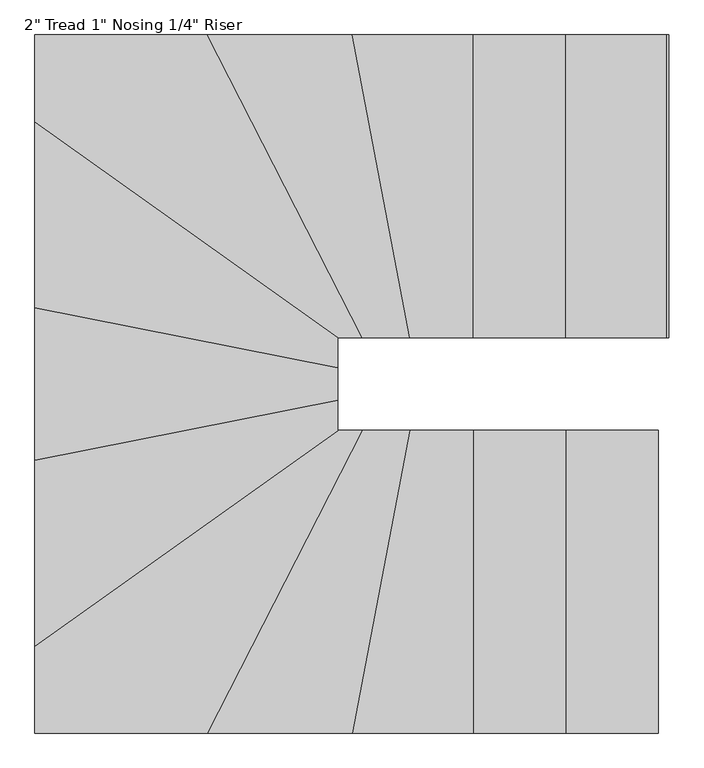
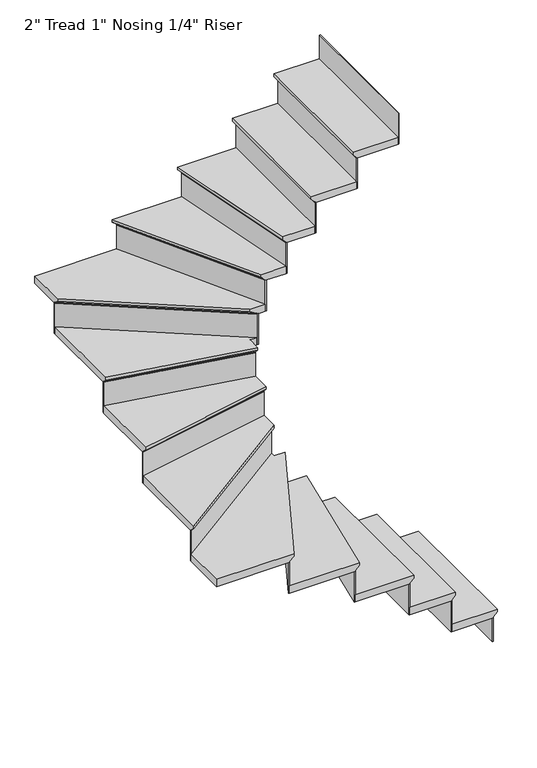
"""IFC4 building model written with IfcOpenShell, lengths in millimetres: stair flight geometry."""

from ifc_helpers import new_model, si_unit, origin, place, context, project, spatial, faceted_brep, source, transform, mapped, element, save


def stair_flight_9fd4ca1a(model_context):
    return source(origin(), model_context, "Body", "Brep", [
        faceted_brep([(-6646.4853347, -3718.0076646, 198.6642857), (-6646.4853347, -3718.0076646, 217.7142857), (-6646.4853347, -4632.4076646, 217.7142857), (-6646.4853347, -4632.4076646, 198.6642857), (-6671.8853347, -3718.0076646, 173.2642857), (-6671.8853347, -4632.4076646, 173.2642857), (-6951.2853347, -3718.0076646, 217.7142857), (-6951.2853347, -4632.4076646, 217.7142857), (-6671.8853347, -4632.4076646, 166.9142857), (-6951.2853347, -4632.4076646, 166.9142857), (-6951.2853347, -3718.0076646, 166.9142857), (-6671.8853347, -3718.0076646, 166.9142857)], [[[0, 1, 2, 3]], [[4, 0, 3, 5]], [[2, 1, 6, 7]], [[8, 9, 10, 11]], [[2, 7, 9, 8, 5, 3]], [[8, 11, 4, 5]], [[6, 1, 0, 4, 11, 10]], [[7, 6, 10, 9]]]),
        faceted_brep([(-6671.8853347, -3718.0076646, 166.9142857), (-6671.8853347, -3718.0076646, 0.0), (-6678.2353347, -3718.0076646, 0.0), (-6678.2353347, -3718.0076646, 166.9142857), (-6671.8853347, -4632.4076646, 166.9142857), (-6678.2353347, -4632.4076646, 166.9142857), (-6678.2353347, -4632.4076646, 0.0), (-6671.8853347, -4632.4076646, 0.0)], [[[0, 1, 2, 3]], [[4, 5, 6, 7]], [[1, 0, 4, 7]], [[2, 1, 7, 6]], [[3, 2, 6, 5]], [[0, 3, 5, 4]]]),
        faceted_brep([(-6951.2853347, -3718.0076646, 384.6285714), (-6951.2853347, -3718.0076646, 166.9142857), (-6957.6353347, -3718.0076646, 166.9142857), (-6957.6353347, -3718.0076646, 384.6285714), (-6951.2853347, -4632.4076646, 384.6285714), (-6957.6353347, -4632.4076646, 384.6285714), (-6957.6353347, -4632.4076646, 166.9142857), (-6951.2853347, -4632.4076646, 166.9142857)], [[[0, 1, 2, 3]], [[4, 5, 6, 7]], [[1, 0, 4, 7]], [[2, 1, 7, 6]], [[3, 2, 6, 5]], [[0, 3, 5, 4]]]),
        faceted_brep([(-6925.8853347, -4632.4076646, 435.4285714), (-6925.8853347, -3718.0076646, 435.4285714), (-7230.6853347, -3718.0076646, 435.4285714), (-7230.6853347, -4632.4076646, 435.4285714), (-6951.2853347, -4632.4076646, 384.6285714), (-7230.6853347, -4632.4076646, 384.6285714), (-7230.6853347, -3718.0076646, 384.6285714), (-6951.2853347, -3718.0076646, 384.6285714), (-6951.2853347, -4632.4076646, 390.9785714), (-6925.8853347, -4632.4076646, 416.3785714), (-6951.2853347, -3718.0076646, 390.9785714), (-6925.8853347, -3718.0076646, 416.3785714)], [[[0, 1, 2, 3]], [[4, 5, 6, 7]], [[0, 3, 5, 4, 8, 9]], [[4, 7, 10, 8]], [[2, 1, 11, 10, 7, 6]], [[3, 2, 6, 5]], [[11, 1, 0, 9]], [[10, 11, 9, 8]]]),
        faceted_brep([(-7230.6853347, -3718.0076646, 602.3428571), (-7230.6853347, -3718.0076646, 384.6285714), (-7237.0353347, -3718.0076646, 384.6285714), (-7237.0353347, -3718.0076646, 602.3428571), (-7230.6853347, -4632.4076646, 602.3428571), (-7237.0353347, -4632.4076646, 602.3428571), (-7237.0353347, -4632.4076646, 384.6285714), (-7230.6853347, -4632.4076646, 384.6285714)], [[[0, 1, 2, 3]], [[4, 5, 6, 7]], [[1, 0, 4, 7]], [[2, 1, 7, 6]], [[3, 2, 6, 5]], [[0, 3, 5, 4]]]),
        faceted_brep([(-7205.2853347, -4632.4076646, 653.1428571), (-7205.2853347, -3718.0076646, 653.1428571), (-7424.0654743, -3718.0076646, 653.1428571), (-7597.0057726, -4632.4076646, 653.1428571), (-7230.6853347, -4632.4076646, 602.3428571), (-7597.0057726, -4632.4076646, 602.3428571), (-7424.0654743, -3718.0076646, 602.3428571), (-7230.6853347, -3718.0076646, 602.3428571), (-7230.6853347, -4632.4076646, 608.6928571), (-7205.2853347, -4632.4076646, 634.0928571), (-7230.6853347, -3718.0076646, 608.6928571), (-7205.2853347, -3718.0076646, 634.0928571)], [[[0, 1, 2, 3]], [[4, 5, 6, 7]], [[0, 3, 5, 4, 8, 9]], [[4, 7, 10, 8]], [[2, 1, 11, 10, 7, 6]], [[3, 2, 6, 5]], [[11, 1, 0, 9]], [[10, 11, 9, 8]]]),
        faceted_brep([(-7424.0654743, -3718.0076646, 820.0571429), (-7424.0654743, -3718.0076646, 602.3428571), (-7430.5280465, -3718.0076646, 602.3428571), (-7430.5280465, -3718.0076646, 820.0571429), (-7597.0057726, -4632.4076646, 820.0571429), (-7603.4683448, -4632.4076646, 820.0571429), (-7603.4683448, -4632.4076646, 602.3428571), (-7597.0057726, -4632.4076646, 602.3428571)], [[[0, 1, 2, 3]], [[4, 5, 6, 7]], [[1, 0, 4, 7]], [[2, 1, 7, 6]], [[3, 2, 6, 5]], [[0, 3, 5, 4]]]),
        faceted_brep([(-7571.1554839, -4632.4076646, 870.8571429), (-7398.2151855, -3718.0076646, 870.8571429), (-7569.6930546, -3718.0076646, 870.8571429), (-8038.5176759, -4632.4076646, 870.8571429), (-7597.0057726, -4632.4076646, 820.0571429), (-8038.5176759, -4632.4076646, 820.0571429), (-7569.6930546, -3718.0076646, 820.0571429), (-7424.0654743, -3718.0076646, 820.0571429), (-7597.0057726, -4632.4076646, 826.4071429), (-7571.1554839, -4632.4076646, 851.8071429), (-7424.0654743, -3718.0076646, 826.4071429), (-7398.2151855, -3718.0076646, 851.8071429)], [[[0, 1, 2, 3]], [[4, 5, 6, 7]], [[0, 3, 5, 4, 8, 9]], [[4, 7, 10, 8]], [[2, 1, 11, 10, 7, 6]], [[3, 2, 6, 5]], [[11, 1, 0, 9]], [[10, 11, 9, 8]]]),
        faceted_brep([(-7569.6930546, -3718.0076646, 1037.7714286), (-7569.6930546, -3718.0076646, 820.0571429), (-7576.8290377, -3718.0076646, 820.0571429), (-7576.8290377, -3718.0076646, 1037.7714286), (-8038.5176759, -4632.4076646, 1037.7714286), (-8045.653659, -4632.4076646, 1037.7714286), (-8045.653659, -4632.4076646, 820.0571429), (-8038.5176759, -4632.4076646, 820.0571429)], [[[0, 1, 2, 3]], [[4, 5, 6, 7]], [[1, 0, 4, 7]], [[2, 1, 7, 6]], [[3, 2, 6, 5]], [[0, 3, 5, 4]]]),
        faceted_brep([(-8529.8170266, -4338.7265309, 1088.5714286), (-8529.8170266, -4632.4076646, 1088.5714286), (-8009.9737433, -4632.4076646, 1088.5714286), (-7541.149122, -3718.0076646, 1088.5714286), (-7615.4170266, -3718.0076646, 1088.5714286), (-7615.4170266, -3688.4525817, 1088.5714286), (-8529.8170266, -4632.4076646, 1037.7714286), (-8529.8170266, -4338.7265309, 1037.7714286), (-7615.4170266, -3688.4525817, 1037.7714286), (-7615.4170266, -3718.0076646, 1037.7714286), (-7569.6930546, -3718.0076646, 1037.7714286), (-8038.5176759, -4632.4076646, 1037.7714286), (-8038.5176759, -4632.4076646, 1044.1214286), (-8009.9737433, -4632.4076646, 1069.5214286), (-7569.6930546, -3718.0076646, 1044.1214286), (-7541.149122, -3718.0076646, 1069.5214286)], [[[0, 1, 2, 3, 4, 5]], [[6, 7, 8, 9, 10, 11]], [[1, 0, 7, 6]], [[2, 1, 6, 11, 12, 13]], [[11, 10, 14, 12]], [[4, 3, 15, 14, 10, 9]], [[5, 4, 9, 8]], [[0, 5, 8, 7]], [[15, 3, 2, 13]], [[14, 15, 13, 12]]]),
        faceted_brep([(-7615.4170266, -3688.4525817, 1255.4857143), (-7615.4170266, -3688.4525817, 1037.7714286), (-7615.4170266, -3680.6606069, 1037.7714286), (-7615.4170266, -3680.6606069, 1255.4857143), (-8529.8170266, -4338.7265309, 1255.4857143), (-8529.8170266, -4330.9345561, 1255.4857143), (-8529.8170266, -4330.9345561, 1037.7714286), (-8529.8170266, -4338.7265309, 1037.7714286)], [[[0, 1, 2, 3]], [[4, 5, 6, 7]], [[1, 0, 4, 7]], [[2, 1, 7, 6]], [[3, 2, 6, 5]], [[0, 3, 5, 4]]]),
        faceted_brep([(-8529.8170266, -4369.8944301, 1306.2857143), (-7615.4170266, -3719.6204809, 1306.2857143), (-7615.4170266, -3601.9984947, 1306.2857143), (-8529.8170266, -3782.239351, 1306.2857143), (-8529.8170266, -4338.7265309, 1255.4857143), (-8529.8170266, -3782.239351, 1255.4857143), (-7615.4170266, -3601.9984947, 1255.4857143), (-7615.4170266, -3688.4525817, 1255.4857143), (-8529.8170266, -4338.7265309, 1261.8357143), (-8529.8170266, -4369.8944301, 1287.2357143), (-7615.4170266, -3688.4525817, 1261.8357143), (-7615.4170266, -3719.6204809, 1287.2357143)], [[[0, 1, 2, 3]], [[4, 5, 6, 7]], [[0, 3, 5, 4, 8, 9]], [[4, 7, 10, 8]], [[2, 1, 11, 10, 7, 6]], [[3, 2, 6, 5]], [[11, 1, 0, 9]], [[10, 11, 9, 8]]]),
        faceted_brep([(-7615.4170266, -3601.9984947, 1473.2), (-7615.4170266, -3601.9984947, 1255.4857143), (-7615.4170266, -3595.5263092, 1255.4857143), (-7615.4170266, -3595.5263092, 1473.2), (-8529.8170266, -3782.239351, 1473.2), (-8529.8170266, -3775.7671656, 1473.2), (-8529.8170266, -3775.7671656, 1255.4857143), (-8529.8170266, -3782.239351, 1255.4857143)], [[[0, 1, 2, 3]], [[4, 5, 6, 7]], [[1, 0, 4, 7]], [[2, 1, 7, 6]], [[3, 2, 6, 5]], [[0, 3, 5, 4]]]),
        faceted_brep([(-8529.8170266, -3808.1280927, 1524.0), (-7615.4170266, -3627.8872364, 1524.0), (-7615.4170266, -3502.839351, 1524.0), (-8529.8170266, -3322.5984947, 1524.0), (-8529.8170266, -3782.239351, 1473.2), (-8529.8170266, -3322.5984947, 1473.2), (-7615.4170266, -3502.839351, 1473.2), (-7615.4170266, -3601.9984947, 1473.2), (-8529.8170266, -3782.239351, 1479.55), (-8529.8170266, -3808.1280927, 1504.95), (-7615.4170266, -3601.9984947, 1479.55), (-7615.4170266, -3627.8872364, 1504.95)], [[[0, 1, 2, 3]], [[4, 5, 6, 7]], [[0, 3, 5, 4, 8, 9]], [[4, 7, 10, 8]], [[2, 1, 11, 10, 7, 6]], [[3, 2, 6, 5]], [[11, 1, 0, 9]], [[10, 11, 9, 8]]]),
        faceted_brep([(-7615.4170266, -3502.839351, 1690.9142857), (-7615.4170266, -3502.839351, 1473.2), (-7615.4170266, -3496.3671656, 1473.2), (-7615.4170266, -3496.3671656, 1690.9142857), (-8529.8170266, -3322.5984947, 1690.9142857), (-8529.8170266, -3316.1263092, 1690.9142857), (-8529.8170266, -3316.1263092, 1473.2), (-8529.8170266, -3322.5984947, 1473.2)], [[[0, 1, 2, 3]], [[4, 5, 6, 7]], [[1, 0, 4, 7]], [[2, 1, 7, 6]], [[3, 2, 6, 5]], [[0, 3, 5, 4]]]),
        faceted_brep([(-8529.8170266, -3348.4872364, 1741.7142857), (-7615.4170266, -3528.7280927, 1741.7142857), (-7615.4170266, -3438.6076646, 1741.7142857), (-7569.3215521, -3438.6076646, 1741.7142857), (-8529.8170266, -2755.5529999, 1741.7142857), (-8529.8170266, -3322.5984947, 1690.9142857), (-8529.8170266, -2755.5529999, 1690.9142857), (-7569.3215521, -3438.6076646, 1690.9142857), (-7615.4170266, -3438.6076646, 1690.9142857), (-7615.4170266, -3502.839351, 1690.9142857), (-8529.8170266, -3322.5984947, 1697.2642857), (-8529.8170266, -3348.4872364, 1722.6642857), (-7615.4170266, -3502.839351, 1697.2642857), (-7615.4170266, -3528.7280927, 1722.6642857)], [[[0, 1, 2, 3, 4]], [[5, 6, 7, 8, 9]], [[0, 4, 6, 5, 10, 11]], [[5, 9, 12, 10]], [[2, 1, 13, 12, 9, 8]], [[3, 2, 8, 7]], [[4, 3, 7, 6]], [[13, 1, 0, 11]], [[12, 13, 11, 10]]]),
        faceted_brep([(-7569.3215521, -3438.6076646, 1908.6285714), (-7569.3215521, -3438.6076646, 1690.9142857), (-7558.3646596, -3438.6076646, 1690.9142857), (-7558.3646596, -3438.6076646, 1908.6285714), (-8529.8170266, -2755.5529999, 1908.6285714), (-8529.8170266, -2747.7610251, 1908.6285714), (-8529.8170266, -2747.7610251, 1690.9142857), (-8529.8170266, -2755.5529999, 1690.9142857)], [[[0, 1, 2, 3]], [[4, 5, 6, 7]], [[1, 0, 4, 7]], [[2, 1, 7, 6]], [[3, 2, 6, 5]], [[0, 3, 5, 4]]]),
        faceted_brep([(-7981.4298108, -2524.2076646, 1959.4285714), (-8529.8170266, -2524.2076646, 1959.4285714), (-8529.8170266, -2786.7208991, 1959.4285714), (-7613.149122, -3438.6076646, 1959.4285714), (-7512.6051895, -3438.6076646, 1959.4285714), (-8529.8170266, -2524.2076646, 1908.6285714), (-7981.4298108, -2524.2076646, 1908.6285714), (-7512.6051895, -3438.6076646, 1908.6285714), (-7569.3215521, -3438.6076646, 1908.6285714), (-8529.8170266, -2755.5529999, 1908.6285714), (-8529.8170266, -2755.5529999, 1914.9785714), (-8529.8170266, -2786.7208991, 1940.3785714), (-7569.3215521, -3438.6076646, 1914.9785714), (-7613.149122, -3438.6076646, 1940.3785714)], [[[0, 1, 2, 3, 4]], [[5, 6, 7, 8, 9]], [[1, 0, 6, 5]], [[2, 1, 5, 9, 10, 11]], [[9, 8, 12, 10]], [[4, 3, 13, 12, 8, 7]], [[0, 4, 7, 6]], [[13, 3, 2, 11]], [[12, 13, 11, 10]]]),
        faceted_brep([(-7512.6051895, -3438.6076646, 2126.3428571), (-7512.6051895, -3438.6076646, 1908.6285714), (-7505.4692064, -3438.6076646, 1908.6285714), (-7505.4692064, -3438.6076646, 2126.3428571), (-7981.4298108, -2524.2076646, 2126.3428571), (-7974.2938277, -2524.2076646, 2126.3428571), (-7974.2938277, -2524.2076646, 1908.6285714), (-7981.4298108, -2524.2076646, 1908.6285714)], [[[0, 1, 2, 3]], [[4, 5, 6, 7]], [[1, 0, 4, 7]], [[2, 1, 7, 6]], [[3, 2, 6, 5]], [[0, 3, 5, 4]]]),
        faceted_brep([(-8009.9737433, -2524.2076646, 2177.1428571), (-7541.149122, -3438.6076646, 2177.1428571), (-7372.3648968, -3438.6076646, 2177.1428571), (-7545.3051951, -2524.2076646, 2177.1428571), (-7981.4298108, -2524.2076646, 2126.3428571), (-7545.3051951, -2524.2076646, 2126.3428571), (-7372.3648968, -3438.6076646, 2126.3428571), (-7512.6051895, -3438.6076646, 2126.3428571), (-7981.4298108, -2524.2076646, 2132.6928571), (-8009.9737433, -2524.2076646, 2158.0928571), (-7512.6051895, -3438.6076646, 2132.6928571), (-7541.149122, -3438.6076646, 2158.0928571)], [[[0, 1, 2, 3]], [[4, 5, 6, 7]], [[0, 3, 5, 4, 8, 9]], [[4, 7, 10, 8]], [[2, 1, 11, 10, 7, 6]], [[3, 2, 6, 5]], [[11, 1, 0, 9]], [[10, 11, 9, 8]]]),
        faceted_brep([(-7372.3648968, -3438.6076646, 2344.0571429), (-7372.3648968, -3438.6076646, 2126.3428571), (-7365.9023246, -3438.6076646, 2126.3428571), (-7365.9023246, -3438.6076646, 2344.0571429), (-7545.3051951, -2524.2076646, 2344.0571429), (-7538.8426229, -2524.2076646, 2344.0571429), (-7538.8426229, -2524.2076646, 2126.3428571), (-7545.3051951, -2524.2076646, 2126.3428571)], [[[0, 1, 2, 3]], [[4, 5, 6, 7]], [[1, 0, 4, 7]], [[2, 1, 7, 6]], [[3, 2, 6, 5]], [[0, 3, 5, 4]]]),
        faceted_brep([(-7571.1554839, -2524.2076646, 2394.8571429), (-7398.2151855, -3438.6076646, 2394.8571429), (-7179.8853347, -3438.6076646, 2394.8571429), (-7179.8853347, -2524.2076646, 2394.8571429), (-7545.3051951, -2524.2076646, 2344.0571429), (-7179.8853347, -2524.2076646, 2344.0571429), (-7179.8853347, -3438.6076646, 2344.0571429), (-7372.3648968, -3438.6076646, 2344.0571429), (-7545.3051951, -2524.2076646, 2350.4071429), (-7571.1554839, -2524.2076646, 2375.8071429), (-7372.3648968, -3438.6076646, 2350.4071429), (-7398.2151855, -3438.6076646, 2375.8071429)], [[[0, 1, 2, 3]], [[4, 5, 6, 7]], [[0, 3, 5, 4, 8, 9]], [[4, 7, 10, 8]], [[2, 1, 11, 10, 7, 6]], [[3, 2, 6, 5]], [[11, 1, 0, 9]], [[10, 11, 9, 8]]]),
        faceted_brep([(-7179.8853347, -3438.6076646, 2561.7714286), (-7179.8853347, -3438.6076646, 2344.0571429), (-7173.5353347, -3438.6076646, 2344.0571429), (-7173.5353347, -3438.6076646, 2561.7714286), (-7179.8853347, -2524.2076646, 2561.7714286), (-7173.5353347, -2524.2076646, 2561.7714286), (-7173.5353347, -2524.2076646, 2344.0571429), (-7179.8853347, -2524.2076646, 2344.0571429)], [[[0, 1, 2, 3]], [[4, 5, 6, 7]], [[1, 0, 4, 7]], [[2, 1, 7, 6]], [[3, 2, 6, 5]], [[0, 3, 5, 4]]]),
        faceted_brep([(-7205.2853347, -2524.2076646, 2612.5714286), (-7205.2853347, -3438.6076646, 2612.5714286), (-6900.4853347, -3438.6076646, 2612.5714286), (-6900.4853347, -2524.2076646, 2612.5714286), (-7179.8853347, -2524.2076646, 2561.7714286), (-6900.4853347, -2524.2076646, 2561.7714286), (-6900.4853347, -3438.6076646, 2561.7714286), (-7179.8853347, -3438.6076646, 2561.7714286), (-7179.8853347, -2524.2076646, 2568.1214286), (-7205.2853347, -2524.2076646, 2593.5214286), (-7179.8853347, -3438.6076646, 2568.1214286), (-7205.2853347, -3438.6076646, 2593.5214286)], [[[0, 1, 2, 3]], [[4, 5, 6, 7]], [[0, 3, 5, 4, 8, 9]], [[4, 7, 10, 8]], [[2, 1, 11, 10, 7, 6]], [[3, 2, 6, 5]], [[11, 1, 0, 9]], [[10, 11, 9, 8]]]),
        faceted_brep([(-6900.4853347, -3438.6076646, 2779.4857143), (-6900.4853347, -3438.6076646, 2561.7714286), (-6894.1353347, -3438.6076646, 2561.7714286), (-6894.1353347, -3438.6076646, 2779.4857143), (-6900.4853347, -2524.2076646, 2779.4857143), (-6894.1353347, -2524.2076646, 2779.4857143), (-6894.1353347, -2524.2076646, 2561.7714286), (-6900.4853347, -2524.2076646, 2561.7714286)], [[[0, 1, 2, 3]], [[4, 5, 6, 7]], [[1, 0, 4, 7]], [[2, 1, 7, 6]], [[3, 2, 6, 5]], [[0, 3, 5, 4]]]),
        faceted_brep([(-6621.0853347, -3438.6076646, 2997.2), (-6621.0853347, -3438.6076646, 2779.4857143), (-6614.7353347, -3438.6076646, 2779.4857143), (-6614.7353347, -3438.6076646, 2997.2), (-6621.0853347, -2524.2076646, 2997.2), (-6614.7353347, -2524.2076646, 2997.2), (-6614.7353347, -2524.2076646, 2779.4857143), (-6621.0853347, -2524.2076646, 2779.4857143)], [[[0, 1, 2, 3]], [[4, 5, 6, 7]], [[1, 0, 4, 7]], [[2, 1, 7, 6]], [[3, 2, 6, 5]], [[0, 3, 5, 4]]]),
        faceted_brep([(-6925.8853347, -2524.2076646, 2830.2857143), (-6925.8853347, -3438.6076646, 2830.2857143), (-6621.0853347, -3438.6076646, 2830.2857143), (-6621.0853347, -2524.2076646, 2830.2857143), (-6900.4853347, -2524.2076646, 2779.4857143), (-6621.0853347, -2524.2076646, 2779.4857143), (-6621.0853347, -3438.6076646, 2779.4857143), (-6900.4853347, -3438.6076646, 2779.4857143), (-6900.4853347, -2524.2076646, 2785.8357143), (-6925.8853347, -2524.2076646, 2811.2357143), (-6900.4853347, -3438.6076646, 2785.8357143), (-6925.8853347, -3438.6076646, 2811.2357143)], [[[0, 1, 2, 3]], [[4, 5, 6, 7]], [[0, 3, 5, 4, 8, 9]], [[4, 7, 10, 8]], [[2, 1, 11, 10, 7, 6]], [[3, 2, 6, 5]], [[11, 1, 0, 9]], [[10, 11, 9, 8]]]),
    ])


if __name__ == "__main__":
    model = new_model("IFC4")
    model_context = context("Model", 3, world=origin())
    ifc_project = project(units=[si_unit("LENGTHUNIT", "METRE", prefix="MILLI")], contexts=[model_context])
    site = spatial("IfcSite", under=ifc_project)
    building = spatial("IfcBuilding", under=site)
    placement = place(None, origin())
    stair_flight_shape = stair_flight_9fd4ca1a(model_context)
    element("IfcStairFlight", 1, ObjectType="2\" Tread 1\" Nosing 1/4\" Riser", at=placement, inside=building, context=model_context, shape_type="MappedRepresentation", body=[
        mapped(stair_flight_shape, transform((0.0, 0.0, 0.0), x_axis=(1.0, 0.0, 0.0), y_axis=(0.0, 1.0, 0.0), z_axis=(0.0, 0.0, 1.0))),
    ])
    save(model, "model.ifc")
